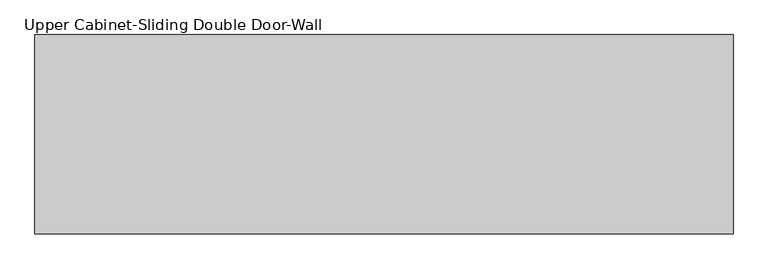
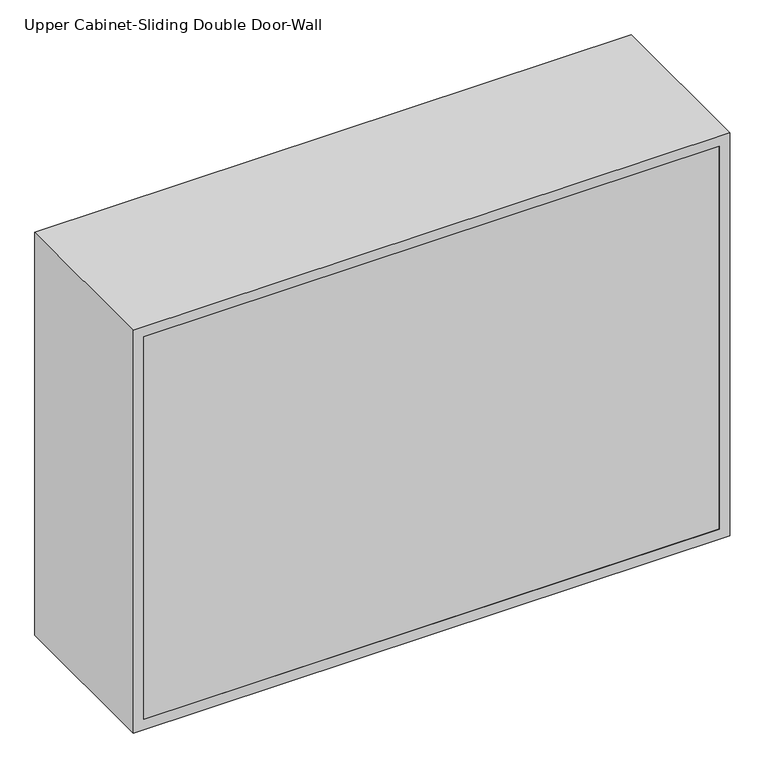
"""IFC4 building model written with IfcOpenShell, lengths in millimetres: furniture geometry, Upper Cabinet-Sliding Double Door-Wall."""

from ifc_helpers import new_model, si_unit, frame, origin, place, context, project, spatial, polyline, outline, extrude, source, transform, mapped, element, save


def upper_cabinet_sliding_double_door_wall_3e092c2a(model_context):
    return source(origin(), model_context, "Body", "SweptSolid", [
        extrude(outline(polyline([(2133.6, -503.6288372), (1371.6, -503.6288372), (1371.6, 563.1711628), (2133.6, 563.1711628), (2133.6, -503.6288372)]), holes=[polyline([(2114.55, -484.5788372), (2114.55, 544.1211628), (1390.65, 544.1211628), (1390.65, -484.5788372), (2114.55, -484.5788372)])]), frame((0.0, 114.3, 0.0), z_axis=(0.0, 1.0, 0.0), x_axis=(0.0, 0.0, 1.0)), (0.0, 0.0, 1.0), 304.8),
        extrude(outline(polyline([(544.1211628, 114.3), (-484.5788372, 114.3), (-484.5788372, 133.35), (544.1211628, 133.35), (544.1211628, 114.3)])), frame((0.0, 0.0, 1390.65), z_axis=(0.0, 0.0, 1.0), x_axis=(1.0, 0.0, 0.0)), (0.0, 0.0, 1.0), 723.9),
        extrude(outline(polyline([(23.4211628, 412.75), (544.1211628, 412.75), (544.1211628, 406.4), (23.4211628, 406.4), (23.4211628, 412.75)])), frame((0.0, 0.0, 1390.65), z_axis=(0.0, 0.0, 1.0), x_axis=(1.0, 0.0, 0.0)), (0.0, 0.0, 1.0), 723.9),
        extrude(outline(polyline([(-484.5788372, 406.4), (36.1211628, 406.4), (36.1211628, 400.05), (-484.5788372, 400.05), (-484.5788372, 406.4)])), frame((0.0, 0.0, 1390.65), z_axis=(0.0, 0.0, 1.0), x_axis=(1.0, 0.0, 0.0)), (0.0, 0.0, 1.0), 723.9),
    ])


if __name__ == "__main__":
    model = new_model("IFC4")
    model_context = context("Model", 3, world=origin())
    ifc_project = project(units=[si_unit("LENGTHUNIT", "METRE", prefix="MILLI")], contexts=[model_context])
    site = spatial("IfcSite", under=ifc_project)
    building = spatial("IfcBuilding", under=site)
    placement = place(None, origin())
    upper_cabinet_sliding_double_door_wall_shape = upper_cabinet_sliding_double_door_wall_3e092c2a(model_context)
    element("IfcFurniture", 1, ObjectType="Upper Cabinet-Sliding Double Door-Wall", at=placement, inside=building, context=model_context, shape_type="MappedRepresentation", body=[
        mapped(upper_cabinet_sliding_double_door_wall_shape, transform((0.0, 0.0, 0.0), x_axis=(1.0, 0.0, 0.0), y_axis=(0.0, 1.0, 0.0), z_axis=(0.0, 0.0, 1.0))),
    ])
    save(model, "model.ifc")

# Revit data of these elements
# Type "Upper Cabinet-Sliding Double Door-Wall"
#   Depth = 1' - 0"
#   Height = 2' - 6"
#   Top Of Cabinet = 7' - 0"
#   Width = 3' - 6"
#   Default Elevation = 0
# Element 1 (IfcFurniture, "Upper Cabinet-Sliding Double Door-Wall")
#   Materials on its faces: "Cabinet", "Glass"
# Materials
#   "Cabinet": colour RGB 204 122 2, transparency 0
#   "Glass": class "Glass", colour RGB 0 128 192, transparency 0.75, Description = "Soda Lime Glass", Cost = 0
